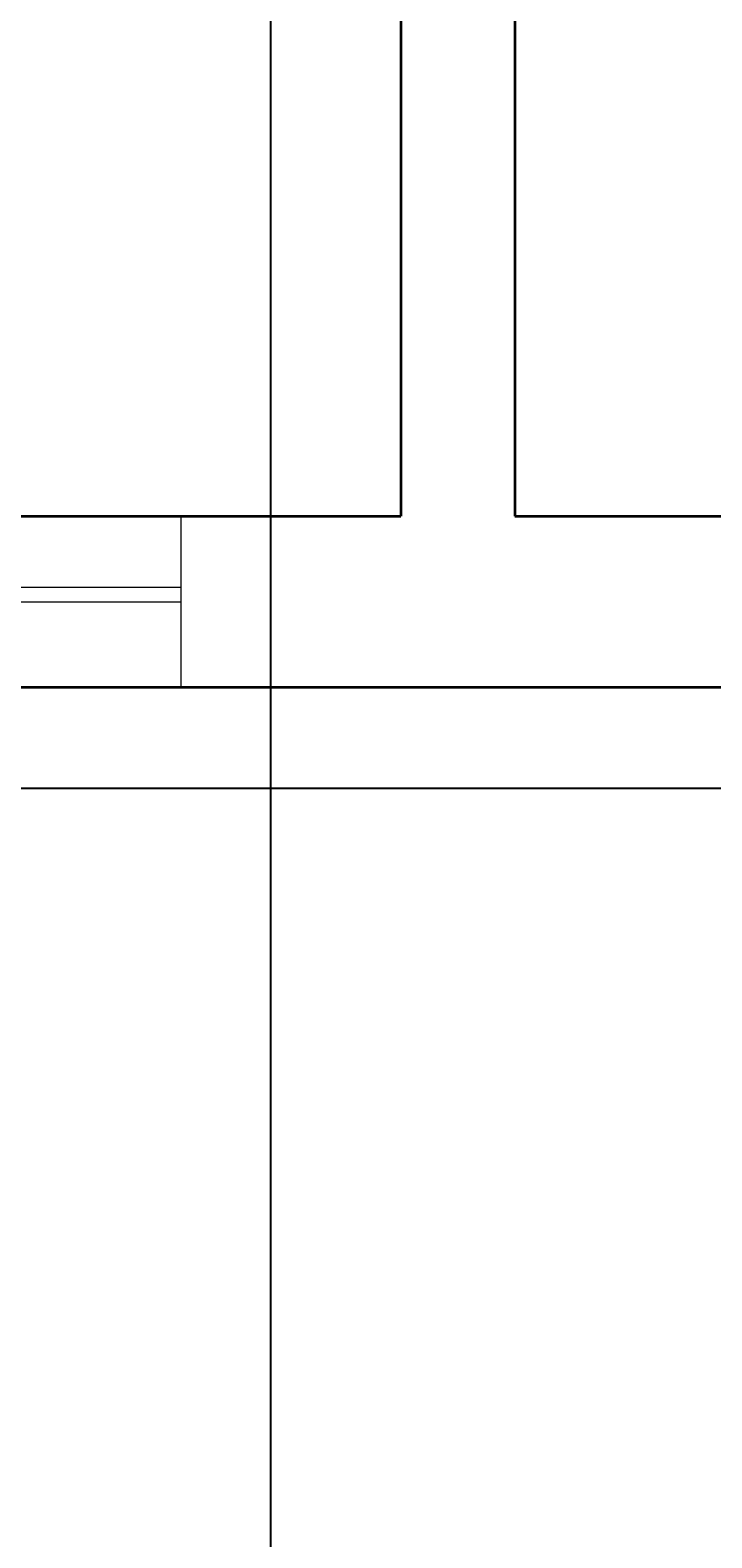
# Model space of a CAD drawing. Units: inches. Extents: x -61 to 1599, y -1316 to 257.
# Tile 78 of 204: x 240 to 276, y -486 to -407. Entities that reach past the tile are written whole.
import ezdxf

# ---------------------------------------------------------------- set-up
doc = ezdxf.new("R2010")
doc.units = ezdxf.units.IN
doc.header["$MEASUREMENT"] = 0
for name, color, linetype, lineweight in [('A-ANNO-DIMS', 2, 'Continuous', 18), ('WALLS', 4, 'Continuous', 35), ('WINDOWS', 220, 'Continuous', 18)]:
    doc.layers.add(name, color=color, linetype=linetype, lineweight=lineweight)
doc.styles.get("Standard").update_dxf_attribs({"font": 'arial.ttf'})
doc.dimstyles.get("Standard").update_dxf_attribs({"dimtxt": 0.18, "dimasz": 0.18, "dimexe": 0.18, "dimexo": 0.0625, "dimgap": 0.09, "dimtad": 0, "dimtih": 1, "dimtoh": 1, "dimdec": 0, "dimzin": 0, "dimdsep": 46, "dimlunit": 3, "dimtxsty": 'Standard', "dimcen": 0.09, "dimadec": 0, "dimazin": 0, "dimtfac": 1, "dimtdec": 0, "dimtofl": 0, "dimtmove": 0, "dimatfit": 3, "dimfxl": 1, "dimtolj": 1, "dimtzin": 0, "dimarcsym": 0})

# ---------------------------------------------------------------- blocks, each defined once
blk = doc.blocks.new('WIN-36IN-2')
for p, q in [((0, 9), (0, 0)), ((36, 9), (36, 0)), ((0, 5.262), (36, 5.262)), ((0, 4.5), (36, 4.5)), ((0, 4.5), (36, 4.5))]:
    blk.add_line(p, q)
blk = doc.blocks.new('*D687')
at = {"layer": 'A-ANNO-DIMS', "color": 0, "lineweight": -2, "transparency": 16777216}
for p, q in [((289.418, 181.677), (-61.077, 181.677)), ((-60.897, 181.497), (-60.897, -528.952)), ((-60.897, -1239.765), (-60.897, -529.316)), ((319.64, -1239.945), (-61.077, -1239.945))]:
    blk.add_line(p, q, dxfattribs=at)
at = {"layer": 'A-ANNO-DIMS', "color": 0, "transparency": 16777216}
for points in [[(-60.927, 181.497), (-60.867, 181.497), (-60.897, 181.677)], [(-60.927, -1239.765), (-60.867, -1239.765), (-60.897, -1239.945)]]:
    blk.add_solid(points, dxfattribs=at)
at = {"layer": 'DEFPOINTS', "color": 0, "transparency": 16777216}
for p in [(289.481, 181.677), (-60.897, -1239.945), (319.703, -1239.945)]:
    blk.add_point(p, dxfattribs=at)
at = {"layer": 'A-ANNO-DIMS', "color": 0, "transparency": 16777216, "insert": (-60.897, -529.134), "char_height": 0.18, "attachment_point": 5}
blk.add_mtext('\\A1;1421.6', dxfattribs=at)
blk = doc.blocks.new('*D699')
at = {"layer": 'A-ANNO-DIMS', "color": 0, "lineweight": -2, "transparency": 16777216}
for p, q in [((835.64, -167.169), (-61.077, -167.169)), ((-60.897, -167.349), (-60.897, -306.726)), ((-60.897, -446.466), (-60.897, -307.09)), ((841.64, -446.646), (-61.077, -446.646))]:
    blk.add_line(p, q, dxfattribs=at)
at = {"layer": 'A-ANNO-DIMS', "color": 0, "transparency": 16777216}
for points in [[(-60.927, -167.349), (-60.867, -167.349), (-60.897, -167.169)], [(-60.927, -446.466), (-60.867, -446.466), (-60.897, -446.646)]]:
    blk.add_solid(points, dxfattribs=at)
at = {"layer": 'DEFPOINTS', "color": 0, "transparency": 16777216}
for p in [(835.703, -167.169), (-60.897, -446.646), (841.703, -446.646)]:
    blk.add_point(p, dxfattribs=at)
at = {"layer": 'A-ANNO-DIMS', "color": 0, "transparency": 16777216, "insert": (-60.897, -306.908), "char_height": 0.18, "attachment_point": 5}
blk.add_mtext('\\A1;279.5', dxfattribs=at)
blk = doc.blocks.new('*D701')
at = {"layer": 'A-ANNO-DIMS', "color": 0, "lineweight": -2, "transparency": 16777216}
for p, q in [((215.752, -616.882), (215.752, 257.457)), ((252.882, -616.882), (252.882, 257.457)), ((215.932, 257.277), (233.924, 257.277)), ((252.702, 257.277), (234.711, 257.277))]:
    blk.add_line(p, q, dxfattribs=at)
at = {"layer": 'A-ANNO-DIMS', "color": 0, "transparency": 16777216}
for points in [[(215.932, 257.307), (215.932, 257.247), (215.752, 257.277)], [(252.702, 257.307), (252.702, 257.247), (252.882, 257.277)]]:
    blk.add_solid(points, dxfattribs=at)
at = {"layer": 'DEFPOINTS', "color": 0, "transparency": 16777216}
for p in [(252.882, 257.277), (215.752, -616.945), (252.882, -616.945)]:
    blk.add_point(p, dxfattribs=at)
at = {"layer": 'A-ANNO-DIMS', "color": 0, "transparency": 16777216, "insert": (234.317, 257.277), "char_height": 0.18, "attachment_point": 5}
blk.add_mtext('\\A1;37.13', dxfattribs=at)

msp = doc.modelspace()

# ---------------------------------------------------------------- linework, layer by layer
at = {"layer": 'WALLS'}
for p, q in [((259.7028, -288.3229), (259.7028, -432.3229)), ((265.7028, -373.3229), (265.7028, -432.3229)), ((237.7028, -432.3229), (259.7028, -432.3229)), ((265.7028, -432.3229), (319.7028, -432.3229)), ((237.7028, -441.3229), (319.7028, -441.3229))]:
    msp.add_line(p, q, dxfattribs=at)

# ---------------------------------------------------------------- block references
at = {"layer": 'WINDOWS'}
msp.add_blockref('WIN-36IN-2', (212.158, -441.323), dxfattribs=at)

# ---------------------------------------------------------------- dimensions: what is measured, and where the dimension line sits
at = {"layer": 'A-ANNO-DIMS'}
dim = msp.add_linear_dim(base=(252.8825, 257.2771), p1=(215.7521, -616.9446), p2=(252.8825, -616.9446), dimstyle='Standard', override={"dimdec": 2, "dimlfac": 1, "dimrnd": 0, "dimzin": 0, "dimdsep": 46, "dimlunit": 2}, dxfattribs=at)
dim.commit()
dim.dimension.update_dxf_attribs({"geometry": '*D701', "text_midpoint": (234.3173, 257.2771)})
for base, p1, p2, picture, middle in [((-60.8972, -1239.9446), (289.4807, 181.6771), (319.7028, -1239.9446), '*D687', (-60.8972, -529.1337)), ((-60.8972, -446.6462), (835.7028, -167.169), (841.7028, -446.6462), '*D699', (-60.8972, -306.9076))]:
    dim = msp.add_linear_dim(base=base, p1=p1, p2=p2, angle=90, dimstyle='Standard', override={"dimdec": 1, "dimlfac": 1, "dimrnd": 0, "dimzin": 0, "dimdsep": 46, "dimlunit": 2}, dxfattribs=at)
    dim.commit()
    dim.dimension.update_dxf_attribs({"geometry": picture, "text_midpoint": middle})

doc.saveas('drawing.dxf')
